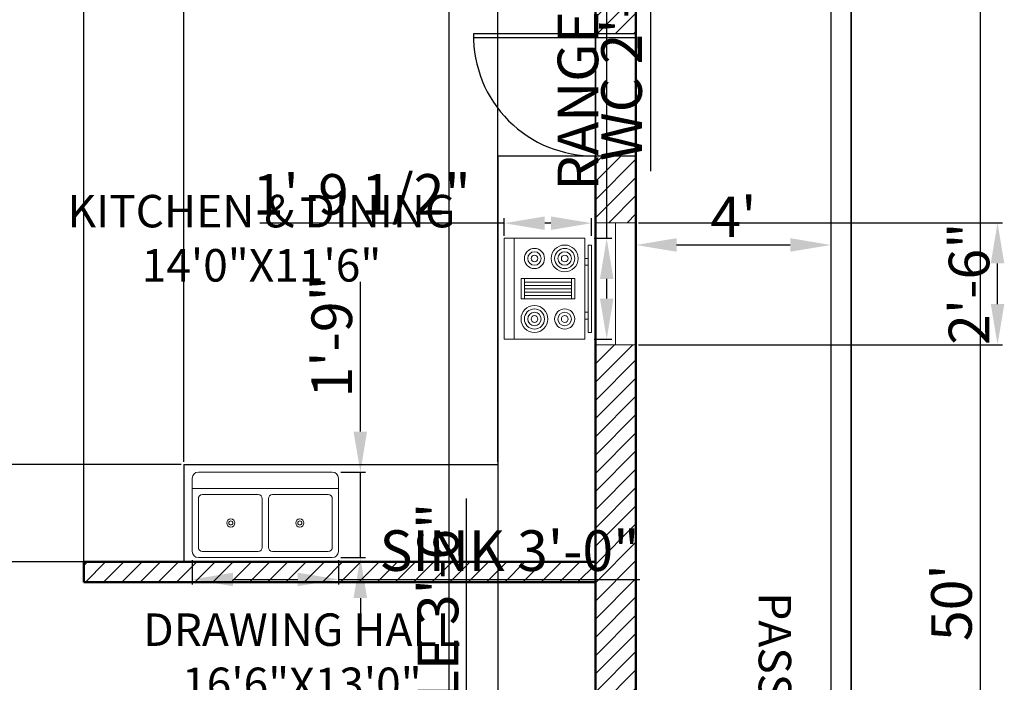
# Model space of a CAD drawing. Units: inches. Extents: x 2206 to 2843, y 1750 to 2489.
# Tile 7 of 8: x 2506 to 2748, y 2075 to 2238. Entities that reach past the tile are written whole.
import ezdxf

# ---------------------------------------------------------------- set-up
doc = ezdxf.new("R2010")
doc.units = ezdxf.units.IN
for name, color, linetype, lineweight in [('A-ANNO-DIMS', 2, 'Continuous', 18), ('A-AREA-IDEN', 7, 'Continuous', 18), ('A-DOOR', 3, 'Continuous', 25), ('A-EQPM', 8, 'Continuous', 18), ('A-FLOR-CASE', 8, 'Continuous', 25), ('A-FLOR-FIXT', 9, 'Continuous', 18), ('A-GLAZ', 4, 'Continuous', 18), ('A-WALL', 7, 'Continuous', 50), ('A-WALL-PATT', 252, 'Continuous', 13), ('C-PROP', 7, 'Continuous', 35), ('L-SITE-WALL', 8, 'Continuous', 25)]:
    doc.layers.add(name, color=color, linetype=linetype, lineweight=lineweight)
doc.styles.get("Standard").update_dxf_attribs({"font": 'arial.ttf'})
doc.dimstyles.new('ISO-25', dxfattribs={"dimtxt": 10, "dimasz": 10, "dimexe": 1.25, "dimexo": 0.625, "dimtad": 1, "dimdec": 1, "dimlunit": 3, "dimtxsty": 'Standard', "dimcen": 2.5, "dimadec": 0, "dimazin": 0, "dimtfac": 1, "dimtdec": 1, "dimtmove": 0, "dimatfit": 3, "dimfxl": 1, "dimarcsym": 0})

# ---------------------------------------------------------------- blocks, each defined once
blk = doc.blocks.new('Range-Oven - 30 in top')
for p, q in [((0, -3), (30, -3)), ((12, -6), (18, -6)), ((13, -20), (13, -6)), ((14, -6), (14, -20)), ((15, -20), (15, -6)), ((16, -6), (16, -20)), ((17, -20), (17, -6)), ((18, -20), (12, -20)), ((6, -24), (6, -25)), ((8, -25), (8, -24)), ((22, -25), (22, -24)), ((24, -24), (24, -25))]:
    blk.add_line(p, q)
for points in [[(0, -24), (0, 0), (30, 0), (30, -24)], [(12, -21), (12, -5), (18, -5), (18, -21)], [(2, -26), (2, -25), (28, -25), (28, -26)]]:
    blk.add_lwpolyline(points, close=True)
for centre, radius in [((6, -9), 4), ((6, -9), 3), ((6, -9), 2), ((6, -9), 1), ((24, -9), 3), ((24, -9), 2), ((24, -9), 1), ((24, -18), 4), ((6, -18), 3), ((6, -18), 2), ((6, -18), 1), ((24, -18), 3), ((24, -18), 2), ((24, -18), 1)]:
    blk.add_circle(centre, radius)
blk = doc.blocks.new('Sink-double - 36 in top')
for p, q in [((-18, -4), (18, -4)), ((-0.75, -18.5), (-0.75, -6.5)), ((0.75, -6.5), (0.75, -18.5))]:
    blk.add_line(p, q)
for points in [[(-16.5, 0), (16.5, 0)], [(-18, -19.5), (-18, -1.5)], [(18, -1.5), (18, -19.5)], [(-16.5, -18.5), (-16.5, -6.5)], [(-15.5, -5.5), (-1.75, -5.5)], [(1.75, -5.5), (15.5, -5.5)], [(16.5, -6.5), (16.5, -18.5)], [(16.5, -21), (-16.5, -21)], [(-1.75, -19.5), (-15.5, -19.5)], [(15.5, -19.5), (1.75, -19.5)]]:
    blk.add_lwpolyline(points)
for centre, radius in [((-8.5, -12.5), 1), ((-8.5, -12.5), 0.5), ((8.5, -12.5), 1), ((8.5, -12.5), 0.5)]:
    blk.add_circle(centre, radius)
for centre, radius, start, end in [((-16.5, -1.5), 1.5, 90, 180), ((16.5, -1.5), 1.5, 0, 90), ((-15.5, -6.5), 1, 90, 180), ((-1.75, -6.5), 1, 0, 90), ((1.75, -6.5), 1, 90, 180), ((15.5, -6.5), 1, 0, 90), ((-15.5, -18.5), 1, 180, 270), ((-1.75, -18.5), 1, 270, 0), ((1.75, -18.5), 1, 180, 270), ((15.5, -18.5), 1, 270, 0), ((-16.5, -19.5), 1.5, 180, 270), ((16.5, -19.5), 1.5, 270, 0)]:
    blk.add_arc(centre, radius, start, end)
blk = doc.blocks.new('*D15')
at = {"layer": 'A-ANNO-DIMS', "color": 0, "lineweight": -2, "transparency": 16777216}
for p, q in [((2711.2, 2394.9), (2743.56, 2394.9)), ((2742.31, 2384.9), (2742.31, 1804.9)), ((2711.2, 1794.9), (2743.56, 1794.9))]:
    blk.add_line(p, q, dxfattribs=at)
at = {"layer": 'A-ANNO-DIMS', "color": 0, "transparency": 16777216}
for points in [[(2740.65, 2384.9), (2743.98, 2384.9), (2742.31, 2394.9)], [(2740.65, 1804.9), (2743.98, 1804.9), (2742.31, 1794.9)]]:
    blk.add_solid(points, dxfattribs=at)
at = {"layer": 'Defpoints', "color": 0, "transparency": 16777216}
for p in [(2710.58, 2394.9), (2710.58, 1794.9), (2742.31, 1794.9)]:
    blk.add_point(p, dxfattribs=at)
at = {"layer": 'A-ANNO-DIMS', "color": 0, "transparency": 16777216, "insert": (2736.58, 2094.9), "char_height": 10, "attachment_point": 5, "rotation": 90}
blk.add_mtext("50'", dxfattribs=at)
blk = doc.blocks.new('*D20')
at = {"layer": 'A-ANNO-DIMS', "color": 0, "lineweight": -2, "transparency": 16777216}
for p, q in [((2657.58, 2187.77), (2657.58, 2181.69)), ((2705.58, 2187.77), (2705.58, 2181.69)), ((2667.58, 2182.94), (2695.58, 2182.94))]:
    blk.add_line(p, q, dxfattribs=at)
at = {"layer": 'A-ANNO-DIMS', "color": 0, "transparency": 16777216}
for points in [[(2667.58, 2184.61), (2667.58, 2181.28), (2657.58, 2182.94)], [(2695.58, 2184.61), (2695.58, 2181.28), (2705.58, 2182.94)]]:
    blk.add_solid(points, dxfattribs=at)
at = {"layer": 'Defpoints', "color": 0, "transparency": 16777216}
for p in [(2657.58, 2188.4), (2705.58, 2188.4), (2705.58, 2182.94)]:
    blk.add_point(p, dxfattribs=at)
at = {"layer": 'A-ANNO-DIMS', "color": 0, "transparency": 16777216, "insert": (2681.58, 2188.57), "char_height": 10, "attachment_point": 5}
blk.add_mtext("4'", dxfattribs=at)
blk = doc.blocks.new('*D33')
at = {"layer": 'A-ANNO-DIMS', "color": 0, "lineweight": -2, "transparency": 16777216}
for p, q in [((2665.45, 2333.95), (2659.87, 2333.95)), ((2661.12, 2323.95), (2661.12, 2310.9)), ((2665.45, 2300.9), (2659.87, 2300.9)), ((2661.12, 2300.9), (2661.12, 2201.13))]:
    blk.add_line(p, q, dxfattribs=at)
at = {"layer": 'A-ANNO-DIMS', "color": 0, "transparency": 16777216}
for points in [[(2659.46, 2323.95), (2662.79, 2323.95), (2661.12, 2333.95)], [(2659.46, 2310.9), (2662.79, 2310.9), (2661.12, 2300.9)]]:
    blk.add_solid(points, dxfattribs=at)
at = {"layer": 'Defpoints', "color": 0, "transparency": 16777216}
for p in [(2666.08, 2333.95), (2661.12, 2300.9), (2666.08, 2300.9)]:
    blk.add_point(p, dxfattribs=at)
at = {"layer": 'A-ANNO-DIMS', "color": 0, "transparency": 16777216, "insert": (2655.33, 2246.01), "char_height": 10, "attachment_point": 5, "rotation": 90}
blk.add_mtext('WC 2\'-9" TYP.', dxfattribs=at)
blk = doc.blocks.new('*D49')
at = {"layer": 'A-ANNO-DIMS', "color": 0, "lineweight": -2, "transparency": 16777216}
for p, q in [((2615.85, 2034.34), (2615.85, 2120.57)), ((2610.18, 2034.34), (2617.1, 2034.34)), ((2615.85, 2002.34), (2615.85, 2024.34)), ((2610.18, 1992.34), (2617.1, 1992.34))]:
    blk.add_line(p, q, dxfattribs=at)
at = {"layer": 'A-ANNO-DIMS', "color": 0, "transparency": 16777216}
for points in [[(2614.19, 2024.34), (2617.52, 2024.34), (2615.85, 2034.34)], [(2614.19, 2002.34), (2617.52, 2002.34), (2615.85, 1992.34)]]:
    blk.add_solid(points, dxfattribs=at)
at = {"layer": 'Defpoints', "color": 0, "transparency": 16777216}
for p in [(2609.55, 2034.34), (2615.85, 2034.34), (2609.55, 1992.34)]:
    blk.add_point(p, dxfattribs=at)
at = {"layer": 'A-ANNO-DIMS', "color": 0, "transparency": 16777216, "insert": (2610.12, 2082.46), "char_height": 10, "attachment_point": 5, "rotation": 90}
blk.add_mtext('TABLE 3\'-6"', dxfattribs=at)
blk = doc.blocks.new('*D53')
at = {"layer": 'A-ANNO-DIMS', "color": 0, "lineweight": -2, "transparency": 16777216}
for p, q in [((2650.37, 2184.58), (2650.37, 2275.46)), ((2647.27, 2184.58), (2651.62, 2184.58)), ((2650.37, 2169.75), (2650.37, 2174.58)), ((2647.27, 2159.75), (2651.62, 2159.75))]:
    blk.add_line(p, q, dxfattribs=at)
at = {"layer": 'A-ANNO-DIMS', "color": 0, "transparency": 16777216}
for points in [[(2648.71, 2174.58), (2652.04, 2174.58), (2650.37, 2184.58)], [(2648.71, 2169.75), (2652.04, 2169.75), (2650.37, 2159.75)]]:
    blk.add_solid(points, dxfattribs=at)
at = {"layer": 'Defpoints', "color": 0, "transparency": 16777216}
for p in [(2646.65, 2184.58), (2650.37, 2184.58), (2646.65, 2159.75)]:
    blk.add_point(p, dxfattribs=at)
at = {"layer": 'A-ANNO-DIMS', "color": 0, "transparency": 16777216, "insert": (2644.58, 2235.02), "char_height": 10, "attachment_point": 5, "rotation": 90}
blk.add_mtext('RANGE 2\'-1"', dxfattribs=at)
blk = doc.blocks.new('*D54')
at = {"layer": 'A-ANNO-DIMS', "color": 0, "lineweight": -2, "transparency": 16777216}
for p, q in [((2625.13, 2188.31), (2564.93, 2188.31)), ((2625.13, 2185.21), (2625.13, 2189.56)), ((2636.65, 2188.31), (2635.13, 2188.31)), ((2646.65, 2185.21), (2646.65, 2189.56))]:
    blk.add_line(p, q, dxfattribs=at)
at = {"layer": 'A-ANNO-DIMS', "color": 0, "transparency": 16777216}
for points in [[(2635.13, 2189.97), (2635.13, 2186.64), (2625.13, 2188.31)], [(2636.65, 2189.97), (2636.65, 2186.64), (2646.65, 2188.31)]]:
    blk.add_solid(points, dxfattribs=at)
at = {"layer": 'Defpoints', "color": 0, "transparency": 16777216}
for p in [(2625.13, 2188.31), (2625.13, 2184.58), (2646.65, 2184.58)]:
    blk.add_point(p, dxfattribs=at)
at = {"layer": 'A-ANNO-DIMS', "color": 0, "transparency": 16777216, "insert": (2590.03, 2194.1), "char_height": 10, "attachment_point": 5}
blk.add_mtext('1\'-9 1/2"', dxfattribs=at)
blk = doc.blocks.new('*D55')
at = {"layer": 'A-ANNO-DIMS', "color": 0, "lineweight": -2, "transparency": 16777216}
for p, q in [((2548.3, 2105.38), (2548.3, 2099.36)), ((2584.3, 2105.38), (2584.3, 2099.36)), ((2558.3, 2100.61), (2574.3, 2100.61)), ((2584.3, 2100.61), (2658.57, 2100.61))]:
    blk.add_line(p, q, dxfattribs=at)
at = {"layer": 'A-ANNO-DIMS', "color": 0, "transparency": 16777216}
for points in [[(2558.3, 2102.27), (2558.3, 2098.94), (2548.3, 2100.61)], [(2574.3, 2102.27), (2574.3, 2098.94), (2584.3, 2100.61)]]:
    blk.add_solid(points, dxfattribs=at)
at = {"layer": 'Defpoints', "color": 0, "transparency": 16777216}
for p in [(2548.3, 2106.01), (2584.3, 2106.01), (2584.3, 2100.61)]:
    blk.add_point(p, dxfattribs=at)
at = {"layer": 'A-ANNO-DIMS', "color": 0, "transparency": 16777216, "insert": (2626.43, 2106.41), "char_height": 10, "attachment_point": 5}
blk.add_mtext('SINK 3\'-0"', dxfattribs=at)
blk = doc.blocks.new('*D56')
at = {"layer": 'A-ANNO-DIMS', "color": 0, "lineweight": -2, "transparency": 16777216}
for p, q in [((2589.7, 2137.01), (2589.7, 2173.9)), ((2584.92, 2127.01), (2590.95, 2127.01)), ((2589.7, 2106.01), (2589.7, 2127.01)), ((2584.92, 2106.01), (2590.95, 2106.01)), ((2589.7, 2096.01), (2589.7, 2086.01))]:
    blk.add_line(p, q, dxfattribs=at)
at = {"layer": 'A-ANNO-DIMS', "color": 0, "transparency": 16777216}
for points in [[(2588.03, 2137.01), (2591.36, 2137.01), (2589.7, 2127.01)], [(2588.03, 2096.01), (2591.36, 2096.01), (2589.7, 2106.01)]]:
    blk.add_solid(points, dxfattribs=at)
at = {"layer": 'Defpoints', "color": 0, "transparency": 16777216}
for p in [(2584.3, 2127.01), (2589.7, 2127.01), (2584.3, 2106.01)]:
    blk.add_point(p, dxfattribs=at)
at = {"layer": 'A-ANNO-DIMS', "color": 0, "transparency": 16777216, "insert": (2583.96, 2160.45), "char_height": 10, "attachment_point": 5, "rotation": 90}
blk.add_mtext('1\'-9"', dxfattribs=at)
blk = doc.blocks.new('*D61')
at = {"layer": 'A-ANNO-DIMS', "color": 0, "lineweight": -2, "transparency": 16777216}
for p, q in [((2479.58, 2100.52), (2479.58, 2432.2)), ((2489.58, 2430.95), (2511.58, 2430.95)), ((2521.58, 2100.52), (2521.58, 2432.2))]:
    blk.add_line(p, q, dxfattribs=at)
at = {"layer": 'A-ANNO-DIMS', "color": 0, "transparency": 16777216}
for points in [[(2489.58, 2432.62), (2489.58, 2429.28), (2479.58, 2430.95)], [(2511.58, 2432.62), (2511.58, 2429.28), (2521.58, 2430.95)]]:
    blk.add_solid(points, dxfattribs=at)
at = {"layer": 'Defpoints', "color": 0, "transparency": 16777216}
for p in [(2521.58, 2430.95), (2479.58, 2099.9), (2521.58, 2099.9)]:
    blk.add_point(p, dxfattribs=at)
at = {"layer": 'A-ANNO-DIMS', "color": 0, "transparency": 16777216, "insert": (2500.58, 2436.68), "char_height": 10, "attachment_point": 5}
blk.add_mtext('3\'-6"', dxfattribs=at)
blk = doc.blocks.new('*D63')
at = {"layer": 'A-ANNO-DIMS', "color": 0, "lineweight": -2, "transparency": 16777216}
for p, q in [((2647.58, 2246.27), (2647.58, 1757.6)), ((2657.58, 2246.27), (2657.58, 1757.6)), ((2637.58, 1758.85), (2627.58, 1758.85)), ((2647.58, 1758.85), (2657.58, 1758.85)), ((2667.58, 1758.85), (2713.18, 1758.85))]:
    blk.add_line(p, q, dxfattribs=at)
at = {"layer": 'A-ANNO-DIMS', "color": 0, "transparency": 16777216}
for points in [[(2637.58, 1760.52), (2637.58, 1757.18), (2647.58, 1758.85)], [(2667.58, 1760.52), (2667.58, 1757.18), (2657.58, 1758.85)]]:
    blk.add_solid(points, dxfattribs=at)
at = {"layer": 'Defpoints', "color": 0, "transparency": 16777216}
for p in [(2647.58, 2246.9), (2657.58, 2246.9), (2657.58, 1758.85)]:
    blk.add_point(p, dxfattribs=at)
at = {"layer": 'A-ANNO-DIMS', "color": 0, "transparency": 16777216, "insert": (2695.38, 1764.58), "char_height": 10, "attachment_point": 5}
blk.add_mtext('0\'-10"', dxfattribs=at)
blk = doc.blocks.new('*D74')
at = {"layer": 'A-ANNO-DIMS', "color": 0, "lineweight": -2, "transparency": 16777216}
for p, q in [((2611.58, 1856.52), (2611.58, 2432.2)), ((2621.58, 2430.95), (2637.58, 2430.95)), ((2647.58, 1856.52), (2647.58, 2432.2))]:
    blk.add_line(p, q, dxfattribs=at)
at = {"layer": 'A-ANNO-DIMS', "color": 0, "transparency": 16777216}
for points in [[(2621.58, 2432.62), (2621.58, 2429.28), (2611.58, 2430.95)], [(2637.58, 2432.62), (2637.58, 2429.28), (2647.58, 2430.95)]]:
    blk.add_solid(points, dxfattribs=at)
at = {"layer": 'Defpoints', "color": 0, "transparency": 16777216}
for p in [(2647.58, 2430.95), (2611.58, 1855.9), (2647.58, 1855.9)]:
    blk.add_point(p, dxfattribs=at)
at = {"layer": 'A-ANNO-DIMS', "color": 0, "transparency": 16777216, "insert": (2629.58, 2436.68), "char_height": 10, "attachment_point": 5}
blk.add_mtext('3\'-0"', dxfattribs=at)
blk = doc.blocks.new('*D76')
at = {"layer": 'A-ANNO-DIMS', "color": 0, "lineweight": -2, "transparency": 16777216}
for p, q in [((2658.2, 2188.4), (2747.88, 2188.4)), ((2746.63, 2168.4), (2746.63, 2178.4)), ((2658.2, 2158.4), (2747.88, 2158.4))]:
    blk.add_line(p, q, dxfattribs=at)
at = {"layer": 'A-ANNO-DIMS', "color": 0, "transparency": 16777216}
for points in [[(2744.96, 2178.4), (2748.3, 2178.4), (2746.63, 2188.4)], [(2744.96, 2168.4), (2748.3, 2168.4), (2746.63, 2158.4)]]:
    blk.add_solid(points, dxfattribs=at)
at = {"layer": 'Defpoints', "color": 0, "transparency": 16777216}
for p in [(2657.58, 2188.4), (2746.63, 2188.4), (2657.58, 2158.4)]:
    blk.add_point(p, dxfattribs=at)
at = {"layer": 'A-ANNO-DIMS', "color": 0, "transparency": 16777216, "insert": (2740.9, 2173.4), "char_height": 10, "attachment_point": 5, "rotation": 90}
blk.add_mtext('2\'-6"', dxfattribs=at)
blk = doc.blocks.new('*D77')
at = {"layer": 'A-ANNO-DIMS', "color": 0, "lineweight": -2, "transparency": 16777216}
for p, q in [((2623.58, 2204.27), (2623.58, 1757.6)), ((2647.58, 2204.27), (2647.58, 1757.6)), ((2633.58, 1758.85), (2637.58, 1758.85)), ((2647.58, 1758.85), (2685.58, 1758.85))]:
    blk.add_line(p, q, dxfattribs=at)
at = {"layer": 'A-ANNO-DIMS', "color": 0, "transparency": 16777216}
for points in [[(2633.58, 1760.52), (2633.58, 1757.18), (2623.58, 1758.85)], [(2637.58, 1760.52), (2637.58, 1757.18), (2647.58, 1758.85)]]:
    blk.add_solid(points, dxfattribs=at)
at = {"layer": 'Defpoints', "color": 0, "transparency": 16777216}
for p in [(2623.58, 2204.9), (2647.58, 2204.9), (2647.58, 1758.85)]:
    blk.add_point(p, dxfattribs=at)
at = {"layer": 'A-ANNO-DIMS', "color": 0, "transparency": 16777216, "insert": (2671.58, 1764.58), "char_height": 10, "attachment_point": 5}
blk.add_mtext('2\'-0"', dxfattribs=at)
blk = doc.blocks.new('*D78')
at = {"layer": 'A-ANNO-DIMS', "color": 0, "lineweight": -2, "transparency": 16777216}
for p, q in [((2218.53, 2128.9), (2218.53, 2166.9)), ((2545.59, 2128.9), (2217.28, 2128.9)), ((2218.53, 2114.9), (2218.53, 2118.9)), ((2545.59, 2104.9), (2217.28, 2104.9))]:
    blk.add_line(p, q, dxfattribs=at)
at = {"layer": 'A-ANNO-DIMS', "color": 0, "transparency": 16777216}
for points in [[(2216.86, 2118.9), (2220.2, 2118.9), (2218.53, 2128.9)], [(2216.86, 2114.9), (2220.2, 2114.9), (2218.53, 2104.9)]]:
    blk.add_solid(points, dxfattribs=at)
at = {"layer": 'Defpoints', "color": 0, "transparency": 16777216}
for p in [(2218.53, 2128.9), (2546.21, 2128.9), (2546.21, 2104.9)]:
    blk.add_point(p, dxfattribs=at)
at = {"layer": 'A-ANNO-DIMS', "color": 0, "transparency": 16777216, "insert": (2212.8, 2152.9), "char_height": 10, "attachment_point": 5, "rotation": 90}
blk.add_mtext('2\'-0"', dxfattribs=at)
blk = doc.blocks.new('*D79')
at = {"layer": 'A-ANNO-DIMS', "color": 0, "lineweight": -2, "transparency": 16777216}
for p, q in [((2546.21, 2129.52), (2546.21, 2432.2)), ((2556.21, 2430.95), (2613.58, 2430.95)), ((2623.58, 2129.52), (2623.58, 2432.2))]:
    blk.add_line(p, q, dxfattribs=at)
at = {"layer": 'A-ANNO-DIMS', "color": 0, "transparency": 16777216}
for points in [[(2556.21, 2432.62), (2556.21, 2429.28), (2546.21, 2430.95)], [(2613.58, 2432.62), (2613.58, 2429.28), (2623.58, 2430.95)]]:
    blk.add_solid(points, dxfattribs=at)
at = {"layer": 'Defpoints', "color": 0, "transparency": 16777216}
for p in [(2623.58, 2430.95), (2546.21, 2128.9), (2623.58, 2128.9)]:
    blk.add_point(p, dxfattribs=at)
at = {"layer": 'A-ANNO-DIMS', "color": 0, "transparency": 16777216, "insert": (2584.9, 2436.74), "char_height": 10, "attachment_point": 5}
blk.add_mtext('6\'-5 1/2"', dxfattribs=at)

msp = doc.modelspace()

# ---------------------------------------------------------------- hatches: boundary and pattern name
at = {"layer": 'A-WALL-PATT'}
h = msp.add_hatch(dxfattribs=at)
h.set_pattern_fill('ANSI31', color=256)
h.paths.add_polyline_path([(2710.58, 2394.9), (2296.58, 2394.9), (2296.58, 2335.9), (2306.58, 2335.9), (2306.58, 2384.9), (2479.58, 2384.9), (2652.58, 2384.9), (2700.58, 2384.9), (2700.58, 2300.9), (2690.58, 2300.9), (2690.58, 2290.9), (2710.58, 2290.9)])
h.paths.add_polyline_path([(2306.58, 2295.9), (2296.58, 2295.9), (2296.58, 2225.9), (2306.58, 2225.9), (2306.58, 2241.9)])
h.paths.add_polyline_path([(2306.58, 2111.9), (2306.58, 2132.9), (2296.58, 2132.9), (2296.58, 2071.9), (2306.58, 2071.9)])
h.paths.add_polyline_path([(2306.58, 2197.9), (2296.58, 2197.9), (2296.58, 2160.9), (2306.58, 2160.9), (2306.58, 2176.9)])
h.paths.add_polyline_path([(2370.58, 1991.9), (2306.58, 1991.9), (2306.58, 2031.9), (2296.58, 2031.9), (2296.58, 1981.9), (2370.58, 1981.9)])
h.paths.add_polyline_path([(2479.58, 2066.9), (2474.58, 2066.9), (2474.58, 1991.9), (2410.58, 1991.9), (2410.58, 1981.9), (2479.58, 1981.9)])
h.paths.add_polyline_path([(2539.58, 1943.9), (2479.58, 1943.9), (2479.58, 1944.9), (2469.58, 1944.9), (2469.58, 1933.9), (2539.58, 1933.9)])
h.paths.add_polyline_path([(2657.58, 1997.9), (2647.58, 1997.9), (2647.58, 1943.9), (2647.58, 1918.9), (2657.58, 1918.9)])
h.paths.add_polyline_path([(2647.58, 1943.9), (2587.58, 1943.9), (2587.58, 1933.9), (2647.58, 1933.9)])
h.paths.add_polyline_path([(2657.58, 2158.4), (2647.58, 2158.4), (2647.58, 2104.9), (2647.58, 2045.9), (2657.58, 2045.9)])
h.paths.add_polyline_path([(2657.58, 2204.89), (2647.58, 2204.89), (2647.58, 2188.4), (2657.58, 2188.4)])
h.paths.add_polyline_path([(2657.58, 2246.9), (2647.58, 2246.9), (2647.58, 2234.9), (2657.58, 2234.9)])
h.paths.add_polyline_path([(2662.58, 2300.9), (2652.58, 2300.9), (2652.58, 2346.22), (2647.58, 2346.22), (2647.58, 2290.9), (2662.58, 2290.9)])
h.paths.add_polyline_path([(2647.58, 2246.9), (2524.58, 2246.9), (2524.58, 2241.9), (2647.58, 2241.9)])
h.paths.add_polyline_path([(2351.58, 2246.9), (2306.58, 2246.9), (2306.58, 2241.9), (2351.58, 2241.9)])
h.paths.add_polyline_path([(2429.58, 2246.9), (2381.58, 2246.9), (2381.58, 2241.9), (2390.58, 2241.9), (2390.58, 2181.9), (2306.58, 2181.9), (2306.58, 2176.9), (2390.58, 2176.9), (2390.58, 2116.9), (2381.58, 2116.9), (2381.58, 2111.9), (2474.58, 2111.9), (2474.58, 2102.9), (2479.58, 2102.9), (2479.58, 2104.9), (2479.58, 2116.9), (2395.58, 2116.9), (2395.58, 2176.9), (2395.58, 2241.9), (2429.58, 2241.9)])
h.paths.add_polyline_path([(2479.58, 2384.9), (2474.58, 2384.9), (2474.58, 2246.9), (2465.58, 2246.9), (2465.58, 2241.9), (2479.58, 2241.9), (2488.58, 2241.9), (2488.58, 2246.9), (2479.58, 2246.9)])
h.paths.add_polyline_path([(2657.58, 1870.9), (2647.58, 1870.9), (2647.58, 1855.9), (2511.58, 1855.9), (2511.58, 1845.9), (2657.58, 1845.9)])
h = msp.add_hatch(dxfattribs=at)
h.set_pattern_fill('ANSI31', color=256)
h.paths.add_polyline_path([(2647.58, 2104.9), (2521.58, 2104.9), (2521.58, 2099.9), (2647.58, 2099.9)])

# ---------------------------------------------------------------- linework, layer by layer
at = {"layer": 'A-DOOR'}
for p, q in [((2657.58, 2234.9), (2617.58, 2234.9)), ((2657.58, 2233.9), (2617.58, 2233.9)), ((2647.08, 2204.89), (2657.58, 2204.89)), ((2657.08, 2204.89), (2657.58, 2204.89))]:
    msp.add_line(p, q, dxfattribs=at)
msp.add_arc((2647.08, 2234.4), 29.5, 179.029, 270.971, dxfattribs=at)
at = {"layer": 'A-FLOR-CASE'}
for p, q in [((2623.58, 2204.9), (2623.58, 2128.9)), ((2623.58, 2204.9), (2647.58, 2204.89)), ((2546.21, 2128.9), (2623.58, 2128.9)), ((2546.21, 2128.9), (2546.21, 2104.9))]:
    msp.add_line(p, q, dxfattribs=at)
at = {"layer": 'A-GLAZ'}
for p, q in [((2647.58, 2188.4), (2657.58, 2188.4)), ((2652.58, 2188.4), (2652.58, 2158.4)), ((2647.58, 2158.4), (2657.58, 2158.4))]:
    msp.add_line(p, q, dxfattribs=at)
at = {"layer": 'A-WALL'}
for p, q in [((2657.58, 2290.9), (2657.58, 1845.9)), ((2647.58, 2246.9), (2647.58, 2234.9)), ((2647.58, 2204.9), (2647.58, 2104.9)), ((2521.58, 2104.9), (2647.58, 2104.9)), ((2521.58, 2104.9), (2521.58, 2099.9)), ((2647.58, 2104.9), (2647.58, 1943.9)), ((2521.58, 2099.9), (2647.58, 2099.9))]:
    msp.add_line(p, q, dxfattribs=at)
at = {"layer": 'C-PROP'}
msp.add_line((2710.58, 2394.9), (2710.58, 1794.9), dxfattribs=at)
at = {"layer": 'L-SITE-WALL'}
msp.add_line((2705.58, 2290.9), (2705.58, 1799.9), dxfattribs=at)

# ---------------------------------------------------------------- block references
at = {"layer": 'A-EQPM', "xscale": 0.8277605839617583, "yscale": 0.8277605839617583, "zscale": 0.8277605839617583, "rotation": 89.99999999999999}
msp.add_blockref('Range-Oven - 30 in top', (2625.13, 2159.75), dxfattribs=at)
at = {"layer": 'A-FLOR-FIXT'}
msp.add_blockref('Sink-double - 36 in top', (2566.3, 2127.01), dxfattribs=at)

# ---------------------------------------------------------------- texts
at = {"layer": 'A-AREA-IDEN', "char_height": 8, "attachment_point": 1}
for s, width, insert in [('\\pxqc;KITCHEN & DINING\\P14\'0"X11\'6"', 140.852, (2494.93, 2195.27)), ('\\pxqc;DRAWING HALL\\P16\'6"X13\'0"', 91.9993, (2529.31, 2092.24))]:
    msp.add_mtext_dynamic_manual_height_columns(s, width=width, gutter_width=12.5, heights=[0], dxfattribs=dict(at, insert=insert))
at = {"layer": 'A-AREA-IDEN', "insert": (2695.8, 2097.44), "char_height": 8, "attachment_point": 1, "rotation": 270}
msp.add_mtext_dynamic_manual_height_columns('PASSAGE', width=73.3542, gutter_width=12.5, heights=[0], dxfattribs=at)

# ---------------------------------------------------------------- dimensions: what is measured, and where the dimension line sits
at = {"layer": 'A-ANNO-DIMS'}
for base, p1, p2, override, picture, middle in [((2623.58, 2430.95), (2546.21, 2128.9), (2623.58, 2128.9), {"dimdec": 1, "dimlfac": 1, "dimrnd": 0, "dimzin": 1, "dimdsep": 46, "dimlunit": 4, "dimfrac": 2}, '*D79', (2584.9, 2436.74)), ((2521.58, 2430.95), (2479.58, 2099.9), (2521.58, 2099.9), {"dimdec": 1, "dimlfac": 1, "dimrnd": 0, "dimzin": 1, "dimdsep": 46, "dimlunit": 4, "dimfrac": 2}, '*D61', (2500.58, 2436.68)), ((2647.58, 2430.95), (2611.58, 1855.9), (2647.58, 1855.9), {"dimdec": 1, "dimlfac": 1, "dimrnd": 0, "dimzin": 1, "dimdsep": 46, "dimlunit": 4, "dimfrac": 2}, '*D74', (2629.58, 2436.68)), ((2657.58, 1758.85), (2647.58, 2246.9), (2657.58, 2246.9), {"dimdec": 1, "dimlfac": 1, "dimrnd": 0, "dimzin": 1, "dimdsep": 46, "dimlunit": 4, "dimfrac": 2}, '*D63', (2695.38, 1764.58)), ((2647.58, 1758.85), (2623.58, 2204.9), (2647.58, 2204.9), {"dimdec": 1, "dimlfac": 1, "dimrnd": 0, "dimzin": 1, "dimdsep": 46, "dimlunit": 4, "dimfrac": 2}, '*D77', (2671.58, 1764.58)), ((2705.58, 2182.94), (2657.58, 2188.4), (2705.58, 2188.4), {"dimclrd": 0, "dimclre": 0, "dimclrt": 0}, '*D20', (2681.58, 2188.57))]:
    dim = msp.add_linear_dim(base=base, p1=p1, p2=p2, dimstyle='ISO-25', override=override, dxfattribs=at)
    dim.commit()
    dim.dimension.update_dxf_attribs({"geometry": picture, "text_midpoint": middle})
for base, p1, p2, angle, override, picture, middle in [((2742.31, 1794.9), (2710.58, 2394.9), (2710.58, 1794.9), 90, {"dimclrd": 0, "dimclre": 0, "dimclrt": 0}, '*D15', (2736.58, 2094.9)), ((2625.13, 2188.31), (2646.65, 2184.58), (2625.13, 2184.58), 180, {"dimdec": 1, "dimlfac": 1, "dimrnd": 0, "dimzin": 1, "dimdsep": 46, "dimlunit": 4, "dimfrac": 2}, '*D54', (2590.03, 2194.1)), ((2746.63, 2188.4), (2657.58, 2158.4), (2657.58, 2188.4), 90, {"dimdec": 1, "dimlfac": 1, "dimrnd": 0, "dimzin": 1, "dimdsep": 46, "dimlunit": 4, "dimfrac": 2}, '*D76', (2740.9, 2173.4)), ((2589.7, 2127.01), (2584.3, 2106.01), (2584.3, 2127.01), 90, {"dimdec": 1, "dimlfac": 1, "dimrnd": 0, "dimzin": 1, "dimdsep": 46, "dimlunit": 4, "dimfrac": 2}, '*D56', (2583.96, 2160.45)), ((2218.53, 2128.9), (2546.21, 2104.9), (2546.21, 2128.9), 90, {"dimdec": 1, "dimlfac": 1, "dimrnd": 0, "dimzin": 1, "dimdsep": 46, "dimlunit": 4, "dimfrac": 2}, '*D78', (2212.8, 2152.9))]:
    dim = msp.add_linear_dim(base=base, p1=p1, p2=p2, angle=angle, dimstyle='ISO-25', override=override, dxfattribs=at)
    dim.commit()
    dim.dimension.update_dxf_attribs({"geometry": picture, "text_midpoint": middle})
for base, p1, p2, angle, text, picture, middle in [((2661.1228, 2300.8992), (2666.0797, 2333.9455), (2666.0797, 2300.8992), 270, 'WC <> TYP.', '*D33', (2655.3273, 2246.0143)), ((2650.37, 2184.58), (2646.65, 2159.75), (2646.65, 2184.58), 90, 'RANGE <>', '*D53', (2644.58, 2235.02)), ((2615.85, 2034.34), (2609.55, 1992.34), (2609.55, 2034.34), 90, 'TABLE <>', '*D49', (2610.12, 2082.46))]:
    dim = msp.add_linear_dim(base=base, p1=p1, p2=p2, angle=angle, text=text, dimstyle='ISO-25', override={"dimdec": 1, "dimlfac": 1, "dimrnd": 0, "dimzin": 1, "dimdsep": 46, "dimlunit": 4, "dimfrac": 2}, dxfattribs=at)
    dim.commit()
    dim.dimension.update_dxf_attribs({"geometry": picture, "text_midpoint": middle})
dim = msp.add_linear_dim(base=(2584.3, 2100.61), p1=(2548.3, 2106.01), p2=(2584.3, 2106.01), text='SINK <>', dimstyle='ISO-25', override={"dimdec": 1, "dimlfac": 1, "dimrnd": 0, "dimzin": 1, "dimdsep": 46, "dimlunit": 4, "dimfrac": 2}, dxfattribs=at)
dim.commit()
dim.dimension.update_dxf_attribs({"geometry": '*D55', "text_midpoint": (2626.43, 2106.41)})

doc.saveas('drawing.dxf')
